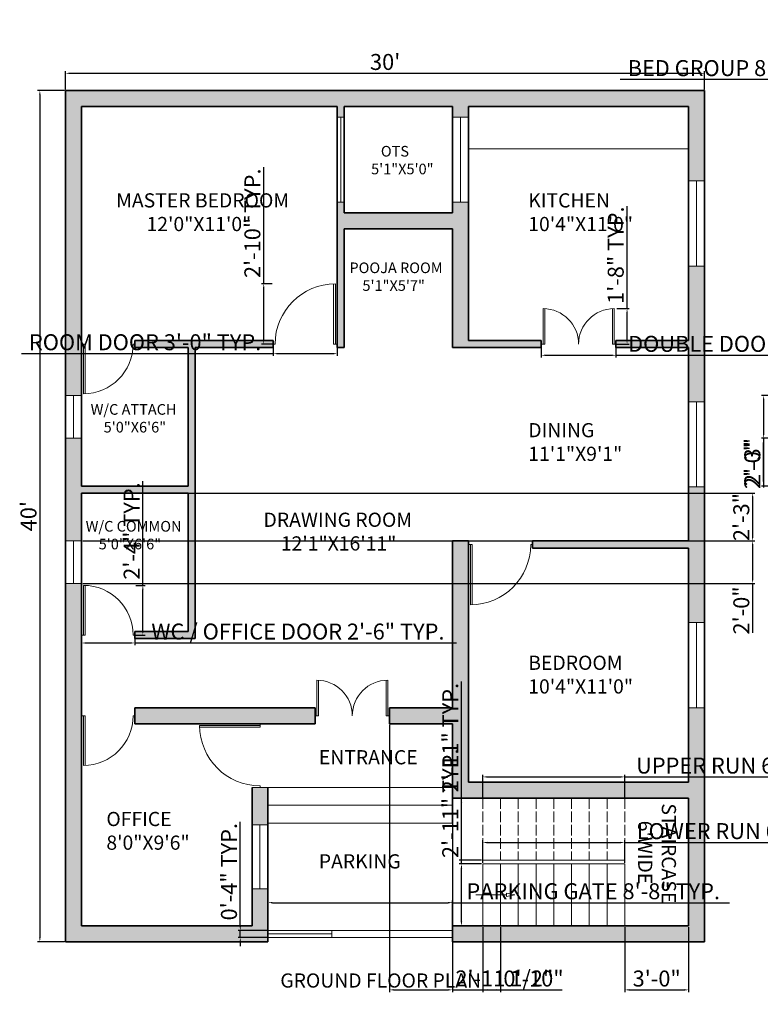
# Model space of a CAD drawing. Units: inches. Extents: x 3592 to 4861, y 1650 to 2243.
# Tile 1 of 30: x 3592 to 4009, y 1650 to 2205. Entities that reach past the tile are written whole.
import ezdxf

# ---------------------------------------------------------------- set-up
doc = ezdxf.new("R2010")
doc.units = ezdxf.units.IN
doc.linetypes.add('ACAD_ISO02W100', pattern=[15, 12, -3])
for name, color, linetype, lineweight in [('A-ANNO-DIMS', 2, 'Continuous', 13), ('A-ANNO-SYMB', 7, 'Continuous', 18), ('A-ANNO-TEXT', 7, 'Continuous', 25), ('A-AREA-IDEN', 7, 'Continuous', 18), ('A-DOOR', 3, 'Continuous', 20), ('A-FLOR-CASE', 7, 'Continuous', 18), ('A-FLOR-STRS', 7, 'Continuous', 18), ('A-FLOR-STRS-OVHD', 8, 'ACAD_ISO02W100', 13), ('A-GLAZ', 4, 'Continuous', 18), ('A-WALL', 7, 'Continuous', 35)]:
    doc.layers.add(name, color=color, linetype=linetype, lineweight=lineweight)
doc.layers.add('A-WALL-PATT', color=252, linetype='Continuous', lineweight=13, true_color=0x939598)
doc.styles.get("Standard").update_dxf_attribs({"font": 'arial.ttf'})
doc.dimstyles.new('ISO-25', dxfattribs={"dimtxt": 9, "dimasz": 2.5, "dimexe": 1.25, "dimexo": 0.625, "dimtad": 1, "dimlunit": 3, "dimtxsty": 'Standard', "dimcen": 2.5, "dimadec": 0, "dimazin": 0, "dimtfac": 1, "dimtmove": 0, "dimatfit": 3, "dimfxl": 1, "dimarcsym": 0})

# ---------------------------------------------------------------- blocks, each defined once
blk = doc.blocks.new('1')
for p, q in [((3628.27, 1890.86), (3628.27, 1924.86)), ((3629.27, 1890.86), (3629.27, 1924.86)), ((3627.27, 1890.86), (3629.27, 1890.86)), ((3662.27, 1890.86), (3663.27, 1890.86))]:
    blk.add_line(p, q)
blk.add_arc((3628.27, 1890.86), 34, 0, 90)
blk = doc.blocks.new('2')
for p, q in [((3637.19, 1914.49), (3637.19, 1942.49)), ((3638.19, 1914.49), (3638.19, 1942.49)), ((3636.19, 1914.49), (3638.19, 1914.49)), ((3665.19, 1914.49), (3666.19, 1914.49))]:
    blk.add_line(p, q)
blk.add_arc((3637.19, 1914.49), 28, 0, 90)
blk = doc.blocks.new('MD')
for p, q in [((3665.34, 1831.69), (3665.34, 1851.69)), ((3666.34, 1831.69), (3666.34, 1851.69)), ((3704.34, 1831.69), (3704.34, 1851.69)), ((3705.34, 1831.69), (3705.34, 1851.69)), ((3664.34, 1831.69), (3666.34, 1831.69)), ((3706.34, 1831.69), (3704.34, 1831.69))]:
    blk.add_line(p, q)
for centre, start, end in [((3665.34, 1831.69), 0, 90), ((3705.34, 1831.69), 90, 180)]:
    blk.add_arc(centre, 20, start, end)
blk = doc.blocks.new('*D4')
at = {"layer": 'A-ANNO-DIMS', "color": 0, "lineweight": -2, "transparency": 16777216}
for p, q in [((3618.06, 2165.84), (3618.06, 2176.13)), ((3978.06, 2165.84), (3978.06, 2176.13)), ((3620.56, 2174.88), (3975.56, 2174.88))]:
    blk.add_line(p, q, dxfattribs=at)
at = {"layer": 'A-ANNO-DIMS', "color": 0, "transparency": 16777216}
for points in [[(3620.56, 2175.3), (3620.56, 2174.46), (3618.06, 2174.88)], [(3975.56, 2175.3), (3975.56, 2174.46), (3978.06, 2174.88)]]:
    blk.add_solid(points, dxfattribs=at)
at = {"layer": 'Defpoints', "color": 0, "transparency": 16777216}
for p in [(3978.06, 2174.88), (3618.06, 2165.22), (3978.06, 2165.22)]:
    blk.add_point(p, dxfattribs=at)
at = {"layer": 'A-ANNO-DIMS', "color": 0, "transparency": 16777216, "insert": (3798.06, 2180.1), "char_height": 9, "attachment_point": 5}
blk.add_mtext("30'", dxfattribs=at)
blk = doc.blocks.new('*D5')
at = {"layer": 'A-ANNO-DIMS', "color": 0, "lineweight": -2, "transparency": 16777216}
for p, q in [((3617.44, 2165.22), (3602.28, 2165.22)), ((3603.53, 2162.72), (3603.53, 1687.72)), ((3617.44, 1685.22), (3602.28, 1685.22))]:
    blk.add_line(p, q, dxfattribs=at)
at = {"layer": 'A-ANNO-DIMS', "color": 0, "transparency": 16777216}
for points in [[(3603.12, 2162.72), (3603.95, 2162.72), (3603.53, 2165.22)], [(3603.12, 1687.72), (3603.95, 1687.72), (3603.53, 1685.22)]]:
    blk.add_solid(points, dxfattribs=at)
at = {"layer": 'Defpoints', "color": 0, "transparency": 16777216}
for p in [(3618.06, 2165.22), (3603.53, 1685.22), (3618.06, 1685.22)]:
    blk.add_point(p, dxfattribs=at)
at = {"layer": 'A-ANNO-DIMS', "color": 0, "transparency": 16777216, "insert": (3598.31, 1925.22), "char_height": 9, "attachment_point": 5, "rotation": 90}
blk.add_mtext("40'", dxfattribs=at)
blk = doc.blocks.new('GATE-PARKING-104')
for p, q in [((104, 4), (0, 4)), ((36, 2), (0, 2)), ((36, 0), (36, 4)), ((104, 0), (0, 0))]:
    blk.add_line(p, q)
blk = doc.blocks.new('ARROW-STAIR-DIRECTION')
blk.add_line((0, 0.94), (17.38, 0.94))
blk.add_lwpolyline([(22.04, 0.94), (17.38, 1.89), (17.38, 0)], close=True)
blk = doc.blocks.new('STAIR-LOWER-RUN')
for p, q in [((0, 35), (80, 35)), ((0, 35), (0, 0)), ((10, 35), (10, 0)), ((20, 35), (20, 0)), ((30, 35), (30, 0)), ((40, 35), (40, 0)), ((50, 35), (50, 0)), ((60, 35), (60, 0)), ((70, 35), (70, 0)), ((80, 35), (80, 0))]:
    blk.add_line(p, q)
blk = doc.blocks.new('STAIR-UPPER-RUN')
at = {"ltscale": 0.5}
for p, q in [((0, 35), (0, 0)), ((10, 35), (10, 0)), ((20, 35), (20, 0)), ((30, 35), (30, 0)), ((40, 35), (40, 0)), ((50, 35), (50, 0)), ((60, 35), (60, 0)), ((70, 35), (70, 0)), ((80, 35), (80, 0))]:
    blk.add_line(p, q, dxfattribs=at)
blk = doc.blocks.new('*D138')
at = {"layer": 'A-ANNO-DIMS', "color": 0, "lineweight": -2, "transparency": 16777216}
for p, q in [((3735.06, 2021.59), (3735.06, 2015.57)), ((3771.06, 2021.59), (3771.06, 2015.57)), ((3735.06, 2016.82), (3593.1, 2016.82)), ((3768.56, 2016.82), (3737.56, 2016.82))]:
    blk.add_line(p, q, dxfattribs=at)
at = {"layer": 'A-ANNO-DIMS', "color": 0, "transparency": 16777216}
for points in [[(3737.56, 2017.24), (3737.56, 2016.4), (3735.06, 2016.82)], [(3768.56, 2017.24), (3768.56, 2016.4), (3771.06, 2016.82)]]:
    blk.add_solid(points, dxfattribs=at)
at = {"layer": 'Defpoints', "color": 0, "transparency": 16777216}
for p in [(3735.06, 2022.22), (3771.06, 2022.22), (3735.06, 2016.82)]:
    blk.add_point(p, dxfattribs=at)
at = {"layer": 'A-ANNO-DIMS', "color": 0, "transparency": 16777216, "insert": (3662.83, 2022.1), "char_height": 9, "attachment_point": 5}
blk.add_mtext('ROOM DOOR 3\'-0" TYP.', dxfattribs=at)
blk = doc.blocks.new('*D139')
at = {"layer": 'A-ANNO-DIMS', "color": 0, "lineweight": -2, "transparency": 16777216}
for p, q in [((3729.66, 2056.22), (3729.66, 2121.97)), ((3734.44, 2056.22), (3728.41, 2056.22)), ((3729.66, 2024.72), (3729.66, 2053.72)), ((3734.44, 2022.22), (3728.41, 2022.22))]:
    blk.add_line(p, q, dxfattribs=at)
at = {"layer": 'A-ANNO-DIMS', "color": 0, "transparency": 16777216}
for points in [[(3729.24, 2053.72), (3730.08, 2053.72), (3729.66, 2056.22)], [(3729.24, 2024.72), (3730.08, 2024.72), (3729.66, 2022.22)]]:
    blk.add_solid(points, dxfattribs=at)
at = {"layer": 'Defpoints', "color": 0, "transparency": 16777216}
for p in [(3729.66, 2056.22), (3735.06, 2056.22), (3735.06, 2022.22)]:
    blk.add_point(p, dxfattribs=at)
at = {"layer": 'A-ANNO-DIMS', "color": 0, "transparency": 16777216, "insert": (3724.44, 2090.35), "char_height": 9, "attachment_point": 5, "rotation": 90}
blk.add_mtext('2\'-10" TYP.', dxfattribs=at)
blk = doc.blocks.new('*D140')
at = {"layer": 'A-ANNO-DIMS', "color": 0, "lineweight": -2, "transparency": 16777216}
for p, q in [((3627.06, 1857.59), (3627.06, 1852.47)), ((3657.06, 1857.59), (3657.06, 1852.47)), ((3629.56, 1853.72), (3654.56, 1853.72)), ((3657.06, 1853.72), (3838.27, 1853.72))]:
    blk.add_line(p, q, dxfattribs=at)
at = {"layer": 'A-ANNO-DIMS', "color": 0, "transparency": 16777216}
for points in [[(3629.56, 1854.14), (3629.56, 1853.3), (3627.06, 1853.72)], [(3654.56, 1854.14), (3654.56, 1853.3), (3657.06, 1853.72)]]:
    blk.add_solid(points, dxfattribs=at)
at = {"layer": 'Defpoints', "color": 0, "transparency": 16777216}
for p in [(3627.06, 1858.22), (3657.06, 1858.22), (3657.06, 1853.72)]:
    blk.add_point(p, dxfattribs=at)
at = {"layer": 'A-ANNO-DIMS', "color": 0, "transparency": 16777216, "insert": (3748.92, 1859), "char_height": 9, "attachment_point": 5}
blk.add_mtext('WC / OFFICE DOOR 2\'-6" TYP.', dxfattribs=at)
blk = doc.blocks.new('*D141')
at = {"layer": 'A-ANNO-DIMS', "color": 0, "lineweight": -2, "transparency": 16777216}
for p, q in [((3661.56, 1886.22), (3661.56, 1944.98)), ((3657.69, 1886.22), (3662.81, 1886.22)), ((3661.56, 1860.72), (3661.56, 1883.72)), ((3657.69, 1858.22), (3662.81, 1858.22))]:
    blk.add_line(p, q, dxfattribs=at)
at = {"layer": 'A-ANNO-DIMS', "color": 0, "transparency": 16777216}
for points in [[(3661.14, 1883.72), (3661.98, 1883.72), (3661.56, 1886.22)], [(3661.14, 1860.72), (3661.98, 1860.72), (3661.56, 1858.22)]]:
    blk.add_solid(points, dxfattribs=at)
at = {"layer": 'Defpoints', "color": 0, "transparency": 16777216}
for p in [(3657.06, 1886.22), (3661.56, 1886.22), (3657.06, 1858.22)]:
    blk.add_point(p, dxfattribs=at)
at = {"layer": 'A-ANNO-DIMS', "color": 0, "transparency": 16777216, "insert": (3656.41, 1916.85), "char_height": 9, "attachment_point": 5, "rotation": 90}
blk.add_mtext('2\'-4" TYP.', dxfattribs=at)
blk = doc.blocks.new('*D142')
at = {"layer": 'A-ANNO-DIMS', "color": 0, "lineweight": -2, "transparency": 16777216}
for p, q in [((3886.06, 2021.59), (3886.06, 2014.67)), ((3928.06, 2021.59), (3928.06, 2014.67)), ((3888.56, 2015.92), (3925.56, 2015.92)), ((3928.06, 2015.92), (4082.63, 2015.92))]:
    blk.add_line(p, q, dxfattribs=at)
at = {"layer": 'A-ANNO-DIMS', "color": 0, "transparency": 16777216}
for points in [[(3888.56, 2016.34), (3888.56, 2015.5), (3886.06, 2015.92)], [(3925.56, 2016.34), (3925.56, 2015.5), (3928.06, 2015.92)]]:
    blk.add_solid(points, dxfattribs=at)
at = {"layer": 'Defpoints', "color": 0, "transparency": 16777216}
for p in [(3886.06, 2022.22), (3928.06, 2022.22), (3928.06, 2015.92)]:
    blk.add_point(p, dxfattribs=at)
at = {"layer": 'A-ANNO-DIMS', "color": 0, "transparency": 16777216, "insert": (4006.6, 2021.2), "char_height": 9, "attachment_point": 5}
blk.add_mtext('DOUBLE DOOR 3\'-6" TYP.', dxfattribs=at)
blk = doc.blocks.new('*D143')
at = {"layer": 'A-ANNO-DIMS', "color": 0, "lineweight": -2, "transparency": 16777216}
for p, q in [((3934.36, 2042.22), (3934.36, 2099.98)), ((3928.69, 2042.22), (3935.61, 2042.22)), ((3934.36, 2024.72), (3934.36, 2039.72)), ((3928.69, 2022.22), (3935.61, 2022.22))]:
    blk.add_line(p, q, dxfattribs=at)
at = {"layer": 'A-ANNO-DIMS', "color": 0, "transparency": 16777216}
for points in [[(3933.94, 2039.72), (3934.78, 2039.72), (3934.36, 2042.22)], [(3933.94, 2024.72), (3934.78, 2024.72), (3934.36, 2022.22)]]:
    blk.add_solid(points, dxfattribs=at)
at = {"layer": 'Defpoints', "color": 0, "transparency": 16777216}
for p in [(3928.06, 2042.22), (3934.36, 2042.22), (3928.06, 2022.22)]:
    blk.add_point(p, dxfattribs=at)
at = {"layer": 'A-ANNO-DIMS', "color": 0, "transparency": 16777216, "insert": (3929.14, 2072.35), "char_height": 9, "attachment_point": 5, "rotation": 90}
blk.add_mtext('1\'-8" TYP.', dxfattribs=at)
blk = doc.blocks.new('*D144')
at = {"layer": 'A-ANNO-DIMS', "color": 0, "lineweight": -2, "transparency": 16777216}
for p, q in [((3732.06, 1692.34), (3732.06, 1708.57)), ((3734.56, 1707.32), (3833.56, 1707.32)), ((3836.06, 1692.34), (3836.06, 1708.57)), ((3836.06, 1707.32), (3992.03, 1707.32))]:
    blk.add_line(p, q, dxfattribs=at)
at = {"layer": 'A-ANNO-DIMS', "color": 0, "transparency": 16777216}
for points in [[(3734.56, 1707.74), (3734.56, 1706.9), (3732.06, 1707.32)], [(3833.56, 1707.74), (3833.56, 1706.9), (3836.06, 1707.32)]]:
    blk.add_solid(points, dxfattribs=at)
at = {"layer": 'Defpoints', "color": 0, "transparency": 16777216}
for p in [(3836.06, 1707.32), (3732.06, 1691.72), (3836.06, 1691.72)]:
    blk.add_point(p, dxfattribs=at)
at = {"layer": 'A-ANNO-DIMS', "color": 0, "transparency": 16777216, "insert": (3915.3, 1712.6), "char_height": 9, "attachment_point": 5}
blk.add_mtext('PARKING GATE 8\'-8" TYP.', dxfattribs=at)
blk = doc.blocks.new('*D145')
at = {"layer": 'A-ANNO-DIMS', "color": 0, "lineweight": -2, "transparency": 16777216}
for p, q in [((3716.46, 1694.22), (3716.46, 1752.83)), ((3731.44, 1691.72), (3715.21, 1691.72)), ((3731.44, 1687.72), (3715.21, 1687.72)), ((3716.46, 1687.72), (3716.46, 1691.72)), ((3716.46, 1685.22), (3716.46, 1682.72))]:
    blk.add_line(p, q, dxfattribs=at)
at = {"layer": 'A-ANNO-DIMS', "color": 0, "transparency": 16777216}
for points in [[(3716.04, 1694.22), (3716.88, 1694.22), (3716.46, 1691.72)], [(3716.04, 1685.22), (3716.88, 1685.22), (3716.46, 1687.72)]]:
    blk.add_solid(points, dxfattribs=at)
at = {"layer": 'Defpoints', "color": 0, "transparency": 16777216}
for p in [(3716.46, 1691.72), (3732.06, 1691.72), (3732.06, 1687.72)]:
    blk.add_point(p, dxfattribs=at)
at = {"layer": 'A-ANNO-DIMS', "color": 0, "transparency": 16777216, "insert": (3711.24, 1724.77), "char_height": 9, "attachment_point": 5, "rotation": 90}
blk.add_mtext('0\'-4" TYP.', dxfattribs=at)
blk = doc.blocks.new('*D146')
at = {"layer": 'A-ANNO-DIMS', "color": 0, "lineweight": -2, "transparency": 16777216}
for p, q in [((3853.06, 1729.84), (3853.06, 1742.47)), ((3855.56, 1741.22), (3930.56, 1741.22)), ((3933.06, 1729.84), (3933.06, 1742.47)), ((3933.06, 1741.22), (4071.6, 1741.22))]:
    blk.add_line(p, q, dxfattribs=at)
at = {"layer": 'A-ANNO-DIMS', "color": 0, "transparency": 16777216}
for points in [[(3855.56, 1741.64), (3855.56, 1740.8), (3853.06, 1741.22)], [(3930.56, 1741.64), (3930.56, 1740.8), (3933.06, 1741.22)]]:
    blk.add_solid(points, dxfattribs=at)
at = {"layer": 'Defpoints', "color": 0, "transparency": 16777216}
for p in [(3933.06, 1741.22), (3853.06, 1729.22), (3933.06, 1729.22)]:
    blk.add_point(p, dxfattribs=at)
at = {"layer": 'A-ANNO-DIMS', "color": 0, "transparency": 16777216, "insert": (4003.58, 1746.5), "char_height": 9, "attachment_point": 5}
blk.add_mtext('LOWER RUN 6\'-8" TYP.', dxfattribs=at)
blk = doc.blocks.new('*D147')
at = {"layer": 'A-ANNO-DIMS', "color": 0, "lineweight": -2, "transparency": 16777216}
for p, q in [((3841.06, 1729.22), (3841.06, 1794.97)), ((3852.44, 1729.22), (3839.81, 1729.22)), ((3841.06, 1696.72), (3841.06, 1726.72)), ((3852.44, 1694.22), (3839.81, 1694.22))]:
    blk.add_line(p, q, dxfattribs=at)
at = {"layer": 'A-ANNO-DIMS', "color": 0, "transparency": 16777216}
for points in [[(3840.64, 1726.72), (3841.48, 1726.72), (3841.06, 1729.22)], [(3840.64, 1696.72), (3841.48, 1696.72), (3841.06, 1694.22)]]:
    blk.add_solid(points, dxfattribs=at)
at = {"layer": 'Defpoints', "color": 0, "transparency": 16777216}
for p in [(3841.06, 1729.22), (3853.06, 1729.22), (3853.06, 1694.22)]:
    blk.add_point(p, dxfattribs=at)
at = {"layer": 'A-ANNO-DIMS', "color": 0, "transparency": 16777216, "insert": (3835.91, 1763.35), "char_height": 9, "attachment_point": 5, "rotation": 90}
blk.add_mtext('2\'-11" TYP.', dxfattribs=at)
blk = doc.blocks.new('*D148')
at = {"layer": 'A-ANNO-DIMS', "color": 0, "lineweight": -2, "transparency": 16777216}
for p, q in [((3853.06, 1766.84), (3853.06, 1779.47)), ((3855.56, 1778.22), (3930.56, 1778.22)), ((3933.06, 1766.84), (3933.06, 1779.47)), ((3933.06, 1778.22), (4068.75, 1778.22))]:
    blk.add_line(p, q, dxfattribs=at)
at = {"layer": 'A-ANNO-DIMS', "color": 0, "transparency": 16777216}
for points in [[(3855.56, 1778.64), (3855.56, 1777.8), (3853.06, 1778.22)], [(3930.56, 1778.64), (3930.56, 1777.8), (3933.06, 1778.22)]]:
    blk.add_solid(points, dxfattribs=at)
at = {"layer": 'Defpoints', "color": 0, "transparency": 16777216}
for p in [(3933.06, 1778.22), (3853.06, 1766.22), (3933.06, 1766.22)]:
    blk.add_point(p, dxfattribs=at)
at = {"layer": 'A-ANNO-DIMS', "color": 0, "transparency": 16777216, "insert": (4002.15, 1783.44), "char_height": 9, "attachment_point": 5}
blk.add_mtext('UPPER RUN 6\'-8" TYP.', dxfattribs=at)
blk = doc.blocks.new('*D149')
at = {"layer": 'A-ANNO-DIMS', "color": 0, "lineweight": -2, "transparency": 16777216}
for p, q in [((3841.06, 1766.22), (3841.06, 1831.97)), ((3852.44, 1766.22), (3839.81, 1766.22)), ((3841.06, 1733.72), (3841.06, 1763.72)), ((3852.44, 1731.22), (3839.81, 1731.22))]:
    blk.add_line(p, q, dxfattribs=at)
at = {"layer": 'A-ANNO-DIMS', "color": 0, "transparency": 16777216}
for points in [[(3840.64, 1763.72), (3841.48, 1763.72), (3841.06, 1766.22)], [(3840.64, 1733.72), (3841.48, 1733.72), (3841.06, 1731.22)]]:
    blk.add_solid(points, dxfattribs=at)
at = {"layer": 'Defpoints', "color": 0, "transparency": 16777216}
for p in [(3841.06, 1766.22), (3853.06, 1766.22), (3853.06, 1731.22)]:
    blk.add_point(p, dxfattribs=at)
at = {"layer": 'A-ANNO-DIMS', "color": 0, "transparency": 16777216, "insert": (3835.91, 1800.35), "char_height": 9, "attachment_point": 5, "rotation": 90}
blk.add_mtext('2\'-11" TYP.', dxfattribs=at)
blk = doc.blocks.new('*D154')
at = {"layer": 'A-ANNO-DIMS', "color": 0, "lineweight": -2, "transparency": 16777216}
for p, q in [((4067.61, 2171.37), (3930.45, 2171.37)), ((4067.61, 2156.84), (4067.61, 2172.62)), ((4166.12, 2171.37), (4070.11, 2171.37)), ((4168.62, 2156.84), (4168.62, 2172.62))]:
    blk.add_line(p, q, dxfattribs=at)
at = {"layer": 'A-ANNO-DIMS', "color": 0, "transparency": 16777216}
for points in [[(4070.11, 2171.79), (4070.11, 2170.95), (4067.61, 2171.37)], [(4166.12, 2171.79), (4166.12, 2170.95), (4168.62, 2171.37)]]:
    blk.add_solid(points, dxfattribs=at)
at = {"layer": 'Defpoints', "color": 0, "transparency": 16777216}
for p in [(4067.61, 2171.37), (4067.61, 2156.22), (4168.62, 2156.22)]:
    blk.add_point(p, dxfattribs=at)
at = {"layer": 'A-ANNO-DIMS', "color": 0, "transparency": 16777216, "insert": (3997.78, 2176.65), "char_height": 9, "attachment_point": 5}
blk.add_mtext('BED GROUP 8\'-5" TYP.', dxfattribs=at)
blk = doc.blocks.new('*D174')
at = {"layer": 'A-ANNO-DIMS', "color": 0, "lineweight": -2, "transparency": 16777216}
for p, q in [((4037.74, 1993.22), (4010.07, 1993.22)), ((4011.32, 1990.72), (4011.32, 1971.72)), ((4037.74, 1969.22), (4010.07, 1969.22)), ((4011.32, 1969.22), (4011.32, 1941.39))]:
    blk.add_line(p, q, dxfattribs=at)
at = {"layer": 'A-ANNO-DIMS', "color": 0, "transparency": 16777216}
for points in [[(4010.9, 1990.72), (4011.74, 1990.72), (4011.32, 1993.22)], [(4010.9, 1971.72), (4011.74, 1971.72), (4011.32, 1969.22)]]:
    blk.add_solid(points, dxfattribs=at)
at = {"layer": 'Defpoints', "color": 0, "transparency": 16777216}
for p in [(4038.37, 1993.22), (4011.32, 1969.22), (4038.37, 1969.22)]:
    blk.add_point(p, dxfattribs=at)
at = {"layer": 'A-ANNO-DIMS', "color": 0, "transparency": 16777216, "insert": (4006.1, 1954.06), "char_height": 9, "attachment_point": 5, "rotation": 90}
blk.add_mtext('2\'-0"', dxfattribs=at)
blk = doc.blocks.new('*D175')
at = {"layer": 'A-ANNO-DIMS', "color": 0, "lineweight": -2, "transparency": 16777216}
for p, q in [((4046.74, 1969.22), (4010.07, 1969.22)), ((4011.32, 1944.72), (4011.32, 1966.72)), ((4046.74, 1942.22), (4010.07, 1942.22))]:
    blk.add_line(p, q, dxfattribs=at)
at = {"layer": 'A-ANNO-DIMS', "color": 0, "transparency": 16777216}
for points in [[(4010.9, 1966.72), (4011.74, 1966.72), (4011.32, 1969.22)], [(4010.9, 1944.72), (4011.74, 1944.72), (4011.32, 1942.22)]]:
    blk.add_solid(points, dxfattribs=at)
at = {"layer": 'Defpoints', "color": 0, "transparency": 16777216}
for p in [(4011.32, 1969.22), (4047.37, 1969.22), (4047.37, 1942.22)]:
    blk.add_point(p, dxfattribs=at)
at = {"layer": 'A-ANNO-DIMS', "color": 0, "transparency": 16777216, "insert": (4006.1, 1955.72), "char_height": 9, "attachment_point": 5, "rotation": 90}
blk.add_mtext('2\'-3"', dxfattribs=at)
blk = doc.blocks.new('*D176')
at = {"layer": 'A-ANNO-DIMS', "color": 0, "lineweight": -2, "transparency": 16777216}
for p, q in [((3627.69, 1938.22), (4006.36, 1938.22)), ((4005.11, 1935.72), (4005.11, 1913.72)), ((3627.69, 1911.22), (4006.36, 1911.22))]:
    blk.add_line(p, q, dxfattribs=at)
at = {"layer": 'A-ANNO-DIMS', "color": 0, "transparency": 16777216}
for points in [[(4004.69, 1935.72), (4005.53, 1935.72), (4005.11, 1938.22)], [(4004.69, 1913.72), (4005.53, 1913.72), (4005.11, 1911.22)]]:
    blk.add_solid(points, dxfattribs=at)
at = {"layer": 'Defpoints', "color": 0, "transparency": 16777216}
for p in [(3627.06, 1938.22), (3627.06, 1911.22), (4005.11, 1911.22)]:
    blk.add_point(p, dxfattribs=at)
at = {"layer": 'A-ANNO-DIMS', "color": 0, "transparency": 16777216, "insert": (3999.89, 1924.72), "char_height": 9, "attachment_point": 5, "rotation": 90}
blk.add_mtext('2\'-3"', dxfattribs=at)
blk = doc.blocks.new('*D177')
at = {"layer": 'A-ANNO-DIMS', "color": 0, "lineweight": -2, "transparency": 16777216}
for p, q in [((3627.69, 1911.22), (4006.36, 1911.22)), ((4005.11, 1908.72), (4005.11, 1889.72)), ((3627.69, 1887.22), (4006.36, 1887.22)), ((4005.11, 1887.22), (4005.11, 1859.39))]:
    blk.add_line(p, q, dxfattribs=at)
at = {"layer": 'A-ANNO-DIMS', "color": 0, "transparency": 16777216}
for points in [[(4004.69, 1908.72), (4005.53, 1908.72), (4005.11, 1911.22)], [(4004.69, 1889.72), (4005.53, 1889.72), (4005.11, 1887.22)]]:
    blk.add_solid(points, dxfattribs=at)
at = {"layer": 'Defpoints', "color": 0, "transparency": 16777216}
for p in [(3627.06, 1911.22), (3627.06, 1887.22), (4005.11, 1887.22)]:
    blk.add_point(p, dxfattribs=at)
at = {"layer": 'A-ANNO-DIMS', "color": 0, "transparency": 16777216, "insert": (3999.89, 1872.06), "char_height": 9, "attachment_point": 5, "rotation": 90}
blk.add_mtext('2\'-0"', dxfattribs=at)
blk = doc.blocks.new('*D180')
at = {"layer": 'A-ANNO-DIMS', "color": 0, "lineweight": -2, "transparency": 16777216}
for p, q in [((3800.56, 1807.59), (3800.56, 1656.92)), ((3836.06, 1807.59), (3836.06, 1656.92)), ((3803.06, 1658.17), (3833.56, 1658.17)), ((3836.06, 1658.17), (3891.85, 1658.17))]:
    blk.add_line(p, q, dxfattribs=at)
at = {"layer": 'A-ANNO-DIMS', "color": 0, "transparency": 16777216}
for points in [[(3803.06, 1658.59), (3803.06, 1657.75), (3800.56, 1658.17)], [(3833.56, 1658.59), (3833.56, 1657.75), (3836.06, 1658.17)]]:
    blk.add_solid(points, dxfattribs=at)
at = {"layer": 'Defpoints', "color": 0, "transparency": 16777216}
for p in [(3800.56, 1808.22), (3836.06, 1808.22), (3836.06, 1658.17)]:
    blk.add_point(p, dxfattribs=at)
at = {"layer": 'A-ANNO-DIMS', "color": 0, "transparency": 16777216, "insert": (3865.21, 1663.45), "char_height": 9, "attachment_point": 5}
blk.add_mtext('2\'-11 1/2"', dxfattribs=at)
blk = doc.blocks.new('*D181')
at = {"layer": 'A-ANNO-DIMS', "color": 0, "lineweight": -2, "transparency": 16777216}
for p, q in [((3933.06, 1693.59), (3933.06, 1656.92)), ((3969.06, 1693.59), (3969.06, 1656.92)), ((3935.56, 1658.17), (3966.56, 1658.17))]:
    blk.add_line(p, q, dxfattribs=at)
at = {"layer": 'A-ANNO-DIMS', "color": 0, "transparency": 16777216}
for points in [[(3935.56, 1658.59), (3935.56, 1657.75), (3933.06, 1658.17)], [(3966.56, 1658.59), (3966.56, 1657.75), (3969.06, 1658.17)]]:
    blk.add_solid(points, dxfattribs=at)
at = {"layer": 'Defpoints', "color": 0, "transparency": 16777216}
for p in [(3933.06, 1694.22), (3969.06, 1694.22), (3969.06, 1658.17)]:
    blk.add_point(p, dxfattribs=at)
at = {"layer": 'A-ANNO-DIMS', "color": 0, "transparency": 16777216, "insert": (3951.06, 1663.39), "char_height": 9, "attachment_point": 5}
blk.add_mtext('3\'-0"', dxfattribs=at)
blk = doc.blocks.new('*D182')
at = {"layer": 'A-ANNO-DIMS', "color": 0, "lineweight": -2, "transparency": 16777216}
for p, q in [((3853.06, 1693.59), (3853.06, 1656.92)), ((3863.06, 1693.59), (3863.06, 1656.92)), ((3855.56, 1658.17), (3860.56, 1658.17)), ((3863.06, 1658.17), (3897.73, 1658.17))]:
    blk.add_line(p, q, dxfattribs=at)
at = {"layer": 'A-ANNO-DIMS', "color": 0, "transparency": 16777216}
for points in [[(3855.56, 1658.59), (3855.56, 1657.75), (3853.06, 1658.17)], [(3860.56, 1658.59), (3860.56, 1657.75), (3863.06, 1658.17)]]:
    blk.add_solid(points, dxfattribs=at)
at = {"layer": 'Defpoints', "color": 0, "transparency": 16777216}
for p in [(3853.06, 1694.22), (3863.06, 1694.22), (3863.06, 1658.17)]:
    blk.add_point(p, dxfattribs=at)
at = {"layer": 'A-ANNO-DIMS', "color": 0, "transparency": 16777216, "insert": (3881.64, 1663.39), "char_height": 9, "attachment_point": 5}
blk.add_mtext('0\'-10"', dxfattribs=at)

msp = doc.modelspace()

# ---------------------------------------------------------------- hatches: boundary and pattern name
at = {"layer": 'A-WALL-PATT'}
h = msp.add_hatch(color=256, dxfattribs=at)
h.dxf.hatch_style = 1
h.paths.add_polyline_path([(3618.061, 2165.219), (3618.061, 1993.219), (3627.061, 1993.219), (3627.061, 2156.219), (3771.061, 2156.219), (3771.061, 2150.219), (3775.061, 2150.219), (3775.061, 2156.219), (3836.061, 2156.219), (3836.061, 2150.219), (3845.061, 2150.219), (3845.061, 2156.219), (3969.061, 2156.219), (3969.061, 2114.219), (3978.061, 2114.219), (3978.061, 2165.219)])
h.paths.add_polyline_path([(3775.061, 2096.219), (3775.061, 2102.219), (3771.061, 2102.219), (3771.061, 2020.219), (3775.061, 2020.219), (3775.061, 2087.219), (3836.061, 2087.219), (3836.061, 2020.219), (3886.061, 2020.219), (3886.061, 2024.219), (3845.061, 2024.219), (3845.061, 2102.219), (3836.061, 2102.219), (3836.061, 2096.219)], flags=17)
h.paths.add_polyline_path([(3969.061, 2024.219), (3928.061, 2024.219), (3928.061, 2020.219), (3969.061, 2020.219), (3969.061, 1989.719), (3978.061, 1989.719), (3978.061, 2066.219), (3969.061, 2066.219)])
h.paths.add_polyline_path([(3969.061, 1865.219), (3978.061, 1865.219), (3978.061, 1941.719), (3969.061, 1941.719), (3969.061, 1911.219), (3881.061, 1911.219), (3881.061, 1907.219), (3969.061, 1907.219)])
h.paths.add_polyline_path([(3978.061, 1817.219), (3969.061, 1817.219), (3969.061, 1775.219), (3845.061, 1775.219), (3845.061, 1911.219), (3836.061, 1911.219), (3836.061, 1817.219), (3800.561, 1817.219), (3800.561, 1808.219), (3836.061, 1808.219), (3836.061, 1766.219), (3969.061, 1766.219), (3969.061, 1694.219), (3836.061, 1694.219), (3836.061, 1685.219), (3978.061, 1685.219)])
h.paths.add_polyline_path([(3657.061, 1817.219), (3657.061, 1808.219), (3758.561, 1808.219), (3758.561, 1817.219)])
h.paths.add_polyline_path([(3691.061, 1856.219), (3691.061, 2020.219), (3735.061, 2020.219), (3735.061, 2024.219), (3657.061, 2024.219), (3657.061, 2020.219), (3687.061, 2020.219), (3687.061, 1942.219), (3627.061, 1942.219), (3627.061, 1969.219), (3618.061, 1969.219), (3618.061, 1911.219), (3627.061, 1911.219), (3627.061, 1938.219), (3687.061, 1938.219), (3687.061, 1860.219), (3657.061, 1860.219), (3657.061, 1856.219)])
h.paths.add_polyline_path([(3627.061, 1887.219), (3618.061, 1887.219), (3618.061, 1685.219), (3732.061, 1685.219), (3732.061, 1715.219), (3723.061, 1715.219), (3723.061, 1694.219), (3627.061, 1694.219)])
h.paths.add_polyline_path([(3723.061, 1751.219), (3732.061, 1751.219), (3732.061, 1772.219), (3723.061, 1772.219)], flags=17)

# ---------------------------------------------------------------- linework, layer by layer
at = {"layer": 'A-FLOR-CASE'}
msp.add_line((3845.061, 2132.219), (3969.061, 2132.219), dxfattribs=at)
at = {"layer": 'A-FLOR-STRS'}
for p, q in [((3836.061, 1772.219), (3723.061, 1772.219)), ((3836.061, 1762.219), (3732.061, 1762.219)), ((3836.061, 1752.219), (3732.061, 1752.219)), ((3853.061, 1731.219), (3933.061, 1731.219))]:
    msp.add_line(p, q, dxfattribs=at)
at = {"layer": 'A-GLAZ'}
for p, q in [((3775.061, 2150.219), (3771.061, 2150.219)), ((3773.061, 2150.219), (3773.061, 2102.219)), ((3845.061, 2150.219), (3836.061, 2150.219)), ((3840.561, 2150.219), (3840.561, 2102.219)), ((3969.061, 2114.219), (3978.061, 2114.219)), ((3973.561, 2114.219), (3973.561, 2066.219)), ((3775.061, 2102.219), (3771.061, 2102.219)), ((3845.061, 2102.219), (3836.061, 2102.219)), ((3969.061, 2066.219), (3978.061, 2066.219)), ((3627.061, 1993.219), (3618.061, 1993.219)), ((3622.561, 1993.219), (3622.561, 1969.219)), ((3969.061, 1989.719), (3978.061, 1989.719)), ((3973.561, 1989.719), (3973.561, 1941.719)), ((3627.061, 1969.219), (3618.061, 1969.219)), ((3969.061, 1941.719), (3978.061, 1941.719)), ((3627.061, 1911.219), (3618.061, 1911.219)), ((3622.561, 1911.219), (3622.561, 1887.219)), ((3627.061, 1887.219), (3618.061, 1887.219)), ((3969.061, 1865.219), (3978.061, 1865.219)), ((3973.561, 1865.219), (3973.561, 1817.219)), ((3969.061, 1817.219), (3978.061, 1817.219)), ((3723.061, 1751.219), (3732.061, 1751.219)), ((3727.561, 1751.219), (3727.561, 1715.219)), ((3723.061, 1715.219), (3732.061, 1715.219))]:
    msp.add_line(p, q, dxfattribs=at)
at = {"layer": 'A-WALL'}
for p, q in [((3618.061, 2165.219), (3978.061, 2165.219)), ((3618.061, 1685.219), (3618.061, 2165.219)), ((3978.061, 2165.219), (3978.061, 1685.219)), ((3627.061, 2156.219), (3771.061, 2156.219)), ((3627.061, 1942.219), (3627.061, 2156.219)), ((3771.061, 2020.219), (3771.061, 2156.219)), ((3775.061, 2156.219), (3836.061, 2156.219)), ((3775.061, 2096.219), (3775.061, 2156.219)), ((3836.061, 2156.219), (3836.061, 2096.219)), ((3845.061, 2156.219), (3845.061, 2024.219)), ((3845.061, 2156.219), (3969.061, 2156.219)), ((3969.061, 2156.219), (3969.061, 2024.219)), ((3775.061, 2096.219), (3836.061, 2096.219)), ((3775.061, 2020.219), (3775.061, 2087.219)), ((3775.061, 2087.219), (3836.061, 2087.219)), ((3836.061, 2087.219), (3836.061, 2020.219)), ((3657.061, 2024.219), (3735.061, 2024.219)), ((3657.061, 2020.219), (3657.061, 2024.219)), ((3735.061, 2020.219), (3735.061, 2024.219)), ((3845.061, 2024.219), (3886.061, 2024.219)), ((3886.061, 2024.219), (3886.061, 2020.219)), ((3928.061, 2024.219), (3928.061, 2020.219)), ((3928.061, 2024.219), (3969.061, 2024.219)), ((3657.061, 2020.219), (3687.061, 2020.219)), ((3687.061, 1942.219), (3687.061, 2020.219)), ((3691.061, 1856.219), (3691.061, 2020.219)), ((3691.061, 2020.219), (3735.061, 2020.219)), ((3771.061, 2020.219), (3775.061, 2020.219)), ((3836.061, 2020.219), (3886.061, 2020.219)), ((3928.061, 2020.219), (3969.061, 2020.219)), ((3969.061, 2020.219), (3969.061, 1911.219)), ((3627.061, 1942.219), (3687.061, 1942.219)), ((3627.061, 1938.219), (3687.061, 1938.219)), ((3627.061, 1694.219), (3627.061, 1938.219)), ((3687.061, 1860.219), (3687.061, 1938.219)), ((3836.061, 1911.219), (3836.061, 1817.219)), ((3845.061, 1911.219), (3836.061, 1911.219)), ((3845.061, 1911.219), (3845.061, 1775.219)), ((3969.061, 1911.219), (3881.061, 1911.219)), ((3881.061, 1911.219), (3881.061, 1907.219)), ((3969.061, 1907.219), (3881.061, 1907.219)), ((3969.061, 1907.219), (3969.061, 1775.219)), ((3657.061, 1860.219), (3687.061, 1860.219)), ((3657.061, 1856.219), (3657.061, 1860.219)), ((3657.061, 1856.219), (3691.061, 1856.219)), ((3657.061, 1808.219), (3657.061, 1817.219)), ((3758.561, 1817.219), (3657.061, 1817.219)), ((3758.561, 1808.219), (3758.561, 1817.219)), ((3836.061, 1817.219), (3800.561, 1817.219)), ((3800.561, 1808.219), (3800.561, 1817.219)), ((3758.561, 1808.219), (3657.061, 1808.219)), ((3836.061, 1808.219), (3800.561, 1808.219)), ((3836.061, 1808.219), (3836.061, 1752.219)), ((3723.061, 1694.219), (3723.061, 1772.219)), ((3732.061, 1685.219), (3732.061, 1772.219)), ((3969.061, 1775.219), (3845.061, 1775.219)), ((3969.061, 1766.219), (3836.061, 1766.219)), ((3969.061, 1766.219), (3969.061, 1694.219)), ((3723.061, 1694.219), (3627.061, 1694.219)), ((3969.061, 1694.219), (3836.061, 1694.219)), ((3836.061, 1694.219), (3836.061, 1685.219)), ((3732.061, 1685.219), (3618.061, 1685.219)), ((3978.061, 1685.219), (3836.061, 1685.219))]:
    msp.add_line(p, q, dxfattribs=at)

# ---------------------------------------------------------------- block references
at = {"layer": 'A-ANNO-SYMB'}
msp.add_blockref('ARROW-STAIR-DIRECTION', (3849.069, 1710.776), dxfattribs=at)
at = {"layer": 'A-DOOR', "xscale": -1}
msp.add_blockref('1', (7398.329, 131.354), dxfattribs=at)
at = {"layer": 'A-DOOR'}
for name, p in [('MD', (221.726, 190.53)), ('2', (-9.128, -56.273)), ('MD', (94.226, -18.97)), ('GATE-PARKING-104', (3732.061, 1687.719))]:
    msp.add_blockref(name, p, dxfattribs=at)
at = {"layer": 'A-DOOR', "xscale": -1}
for name, p, rotation in [('2', (-9.128, 3936.711), 180), ('1', (217.794, 3800.083), 180), ('2', (-9.128, 3727.211), 180), ('1', (5618.426, 5435.486), 90)]:
    msp.add_blockref(name, p, dxfattribs=dict(at, rotation=rotation))
at = {"layer": 'A-FLOR-STRS'}
msp.add_blockref('STAIR-LOWER-RUN', (3853.061, 1694.219), dxfattribs=at)
at = {"layer": 'A-FLOR-STRS-OVHD'}
msp.add_blockref('STAIR-UPPER-RUN', (3853.061, 1731.219), dxfattribs=at)

# ---------------------------------------------------------------- texts
at = {"layer": 'A-ANNO-TEXT', "insert": (3738.994, 1667.444), "char_height": 8, "attachment_point": 1}
msp.add_mtext_dynamic_manual_height_columns('GROUND FLOOR PLAN', width=131.60551, gutter_width=12.5, heights=[0], dxfattribs=at)
at = {"layer": 'A-AREA-IDEN', "attachment_point": 1}
for s, width, insert, char_height in [('   OTS\\P5\'1"X5\'0"', 121.44943, (3790.154, 2133.938), 6), ('MASTER BEDROOM\\P       12\'0"X11\'0"', 121.44943, (3646.522, 2107.241), 8), ('KITCHEN\\P10\'4"X11\'0"', 121.44943, (3878.71, 2107.241), 8), ('POOJA ROOM\\P    5\'1"X5\'7"', 121.44943, (3777.941, 2068.232), 6), ('W/C ATTACH\\P    5\'0"X6\'6"', 121.44943, (3632.145, 1988.392), 6), ('DINING\\P11\'1"X9\'1"', 121.44943, (3878.71, 1977.695), 8), ('DRAWING ROOM\\P    12\'1"X16\'11"', 142.74418, (3729.541, 1927.191), 8), ('W/C COMMON\\P    5\'0"X6\'6"', 121.44943, (3629.34, 1922.501), 6), ('BEDROOM\\P10\'4"X11\'0"', 121.44943, (3878.71, 1846.565), 8), ('ENTRANCE', 121.44943, (3760.707, 1793.311), 8), ('OFFICE\\P8\'0"X9\'6"', 121.44943, (3641.013, 1758.494), 8), ('PARKING', 121.44943, (3760.707, 1734.612), 8)]:
    msp.add_mtext_dynamic_manual_height_columns(s, width=width, gutter_width=12.5, heights=[0], dxfattribs=dict(at, insert=insert, char_height=char_height))
at = {"layer": 'A-AREA-IDEN', "insert": (3961.934, 1763.303), "char_height": 8, "attachment_point": 1, "rotation": 270}
msp.add_mtext_dynamic_manual_height_columns("STAIRCASE\\P    6'WIDE", width=121.44943, gutter_width=12.5, heights=[0], dxfattribs=at)

# ---------------------------------------------------------------- dimensions: what is measured, and where the dimension line sits
at = {"layer": 'A-ANNO-DIMS'}
for base, p1, p2, angle, text, picture, middle in [((4067.606, 2171.371), (4168.621, 2156.219), (4067.606, 2156.219), 180, 'BED GROUP <> TYP.', '*D154', (3997.779, 2176.653)), ((3729.661, 2056.219), (3735.061, 2022.219), (3735.061, 2056.219), 90, '<> TYP.', '*D139', (3724.441, 2090.347)), ((3934.361, 2042.219), (3928.061, 2022.219), (3928.061, 2042.219), 90, '<> TYP.', '*D143', (3929.141, 2072.35)), ((3735.061, 2016.819), (3771.061, 2022.219), (3735.061, 2022.219), 180, 'ROOM DOOR <> TYP.', '*D138', (3662.831, 2022.104)), ((3661.561, 1886.219), (3657.061, 1858.219), (3657.061, 1886.219), 90, '<> TYP.', '*D141', (3656.415, 1916.85)), ((3841.061, 1766.219), (3853.061, 1731.219), (3853.061, 1766.219), 90, '<> TYP.', '*D149', (3835.915, 1800.347)), ((3841.061, 1729.219), (3853.061, 1694.219), (3853.061, 1729.219), 90, '<> TYP.', '*D147', (3835.915, 1763.347)), ((3716.461, 1691.719), (3732.061, 1687.719), (3732.061, 1691.719), 90, '<> TYP.', '*D145', (3711.241, 1724.774))]:
    dim = msp.add_linear_dim(base=base, p1=p1, p2=p2, angle=angle, text=text, dimstyle='ISO-25', override={"dimdec": 1, "dimlfac": 1, "dimrnd": 0, "dimzin": 1, "dimdsep": 46, "dimlunit": 4, "dimfrac": 2}, dxfattribs=at)
    dim.commit()
    dim.dimension.update_dxf_attribs({"geometry": picture, "text_midpoint": middle})
for base, p1, p2, override, picture, middle in [((3978.061, 2174.88), (3618.061, 2165.219), (3978.061, 2165.219), {"dimclrd": 0, "dimclre": 0, "dimclrt": 0}, '*D4', (3798.061, 2180.103)), ((3836.061, 1658.169), (3800.561, 1808.219), (3836.061, 1808.219), {"dimdec": 1, "dimlfac": 1, "dimrnd": 0, "dimzin": 1, "dimdsep": 46, "dimlunit": 4, "dimfrac": 2}, '*D180', (3865.207, 1663.447)), ((3863.061, 1658.169), (3853.061, 1694.219), (3863.061, 1694.219), {"dimdec": 1, "dimlfac": 1, "dimrnd": 0, "dimzin": 1, "dimdsep": 46, "dimlunit": 4, "dimfrac": 2}, '*D182', (3881.645, 1663.389)), ((3969.061, 1658.169), (3933.061, 1694.219), (3969.061, 1694.219), {"dimdec": 1, "dimlfac": 1, "dimrnd": 0, "dimzin": 1, "dimdsep": 46, "dimlunit": 4, "dimfrac": 2}, '*D181', (3951.061, 1663.392))]:
    dim = msp.add_linear_dim(base=base, p1=p1, p2=p2, dimstyle='ISO-25', override=override, dxfattribs=at)
    dim.commit()
    dim.dimension.update_dxf_attribs({"geometry": picture, "text_midpoint": middle})
for base, p1, p2, override, picture, middle in [((3603.534, 1685.219), (3618.061, 2165.219), (3618.061, 1685.219), {"dimclrd": 0, "dimclre": 0, "dimclrt": 0}, '*D5', (3598.314, 1925.219)), ((4011.32, 1969.219), (4038.37, 1993.219), (4038.37, 1969.219), {"dimdec": 1, "dimlfac": 1, "dimrnd": 0, "dimzin": 1, "dimdsep": 46, "dimlunit": 4, "dimfrac": 2}, '*D174', (4006.1, 1954.055)), ((4011.32, 1969.219), (4047.37, 1942.219), (4047.37, 1969.219), {"dimdec": 1, "dimlfac": 1, "dimrnd": 0, "dimzin": 1, "dimdsep": 46, "dimlunit": 4, "dimfrac": 2}, '*D175', (4006.096, 1955.719)), ((4005.111, 1911.219), (3627.061, 1938.219), (3627.061, 1911.219), {"dimdec": 1, "dimlfac": 1, "dimrnd": 0, "dimzin": 1, "dimdsep": 46, "dimlunit": 4, "dimfrac": 2}, '*D176', (3999.888, 1924.719)), ((4005.111, 1887.219), (3627.061, 1911.219), (3627.061, 1887.219), {"dimdec": 1, "dimlfac": 1, "dimrnd": 0, "dimzin": 1, "dimdsep": 46, "dimlunit": 4, "dimfrac": 2}, '*D177', (3999.891, 1872.055))]:
    dim = msp.add_linear_dim(base=base, p1=p1, p2=p2, angle=90, dimstyle='ISO-25', override=override, dxfattribs=at)
    dim.commit()
    dim.dimension.update_dxf_attribs({"geometry": picture, "text_midpoint": middle})
for base, p1, p2, text, picture, middle in [((3928.061, 2015.919), (3886.061, 2022.219), (3928.061, 2022.219), 'DOUBLE DOOR <> TYP.', '*D142', (4006.597, 2021.204)), ((3657.061, 1853.719), (3627.061, 1858.219), (3657.061, 1858.219), 'WC / OFFICE DOOR <> TYP.', '*D140', (3748.915, 1859.001)), ((3933.061, 1778.219), (3853.061, 1766.219), (3933.061, 1766.219), 'UPPER RUN <> TYP.', '*D148', (4002.155, 1783.439)), ((3933.061, 1741.219), (3853.061, 1729.219), (3933.061, 1729.219), 'LOWER RUN <> TYP.', '*D146', (4003.582, 1746.501)), ((3836.061, 1707.319), (3732.061, 1691.719), (3836.061, 1691.719), 'PARKING GATE <> TYP.', '*D144', (3915.296, 1712.597))]:
    dim = msp.add_linear_dim(base=base, p1=p1, p2=p2, text=text, dimstyle='ISO-25', override={"dimdec": 1, "dimlfac": 1, "dimrnd": 0, "dimzin": 1, "dimdsep": 46, "dimlunit": 4, "dimfrac": 2}, dxfattribs=at)
    dim.commit()
    dim.dimension.update_dxf_attribs({"geometry": picture, "text_midpoint": middle})

doc.saveas('drawing.dxf')
